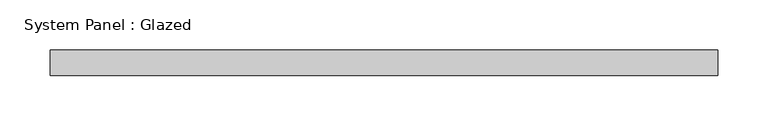
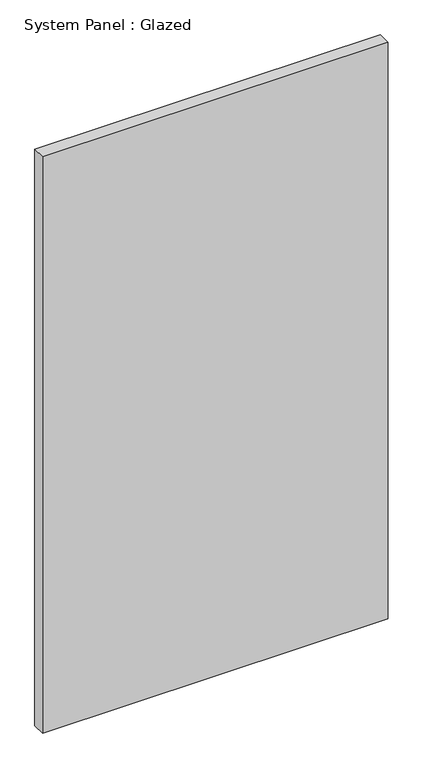
"""IFC4 building model written with IfcOpenShell, lengths in millimetres: plate geometry, System Panel : Glazed."""

from ifc_helpers import new_model, si_unit, origin, origin_with_axes, place, context, project, spatial, polyline, outline, extrude, source, transform, mapped, element, save


def system_panel_glazed_d181f412(model_context):
    return source(origin(), model_context, "Body", "SweptSolid", [
        extrude(outline(polyline([(332.3166667, 19.05), (-332.3166667, 19.05), (-332.3166667, 44.45), (332.3166667, 44.45), (332.3166667, 19.05)])), origin_with_axes(), (0.0, 0.0, 1.0), 1171.2581531),
    ])


if __name__ == "__main__":
    model = new_model("IFC4")
    model_context = context("Model", 3, world=origin())
    ifc_project = project(units=[si_unit("LENGTHUNIT", "METRE", prefix="MILLI")], contexts=[model_context])
    site = spatial("IfcSite", under=ifc_project)
    building = spatial("IfcBuilding", under=site)
    placement = place(None, origin())
    system_panel_glazed_shape = system_panel_glazed_d181f412(model_context)
    element("IfcPlate", 1, ObjectType="System Panel : Glazed", at=placement, inside=building, context=model_context, shape_type="MappedRepresentation", body=[
        mapped(system_panel_glazed_shape, transform((0.0, 0.0, 0.0), x_axis=(1.0, 0.0, 0.0), y_axis=(0.0, 1.0, 0.0), z_axis=(0.0, 0.0, 1.0))),
    ])
    save(model, "model.ifc")

# Revit data of these elements
# Type "System Panel : Glazed"
#   Construction Type Id = "GSP4R"
#   Analytic Construction = "1/8 in Pilkington single glazing"
#   Visual Light Transmittance = 0.9
#   Solar Heat Gain Coefficient = 0.86
#   Heat Transfer Coefficient (U) = 1.18115 BTU/(h·ft²·°F)
#   Define Thermal Properties by = 1
# Element 1 (IfcPlate, "System Panel : Glazed")
#   Materials on its faces: "Glass"
# Materials
#   "Glass": class "Glass", colour RGB 0 128 192, transparency 0.75, Description = "Soda Lime Glass", Cost = 0
